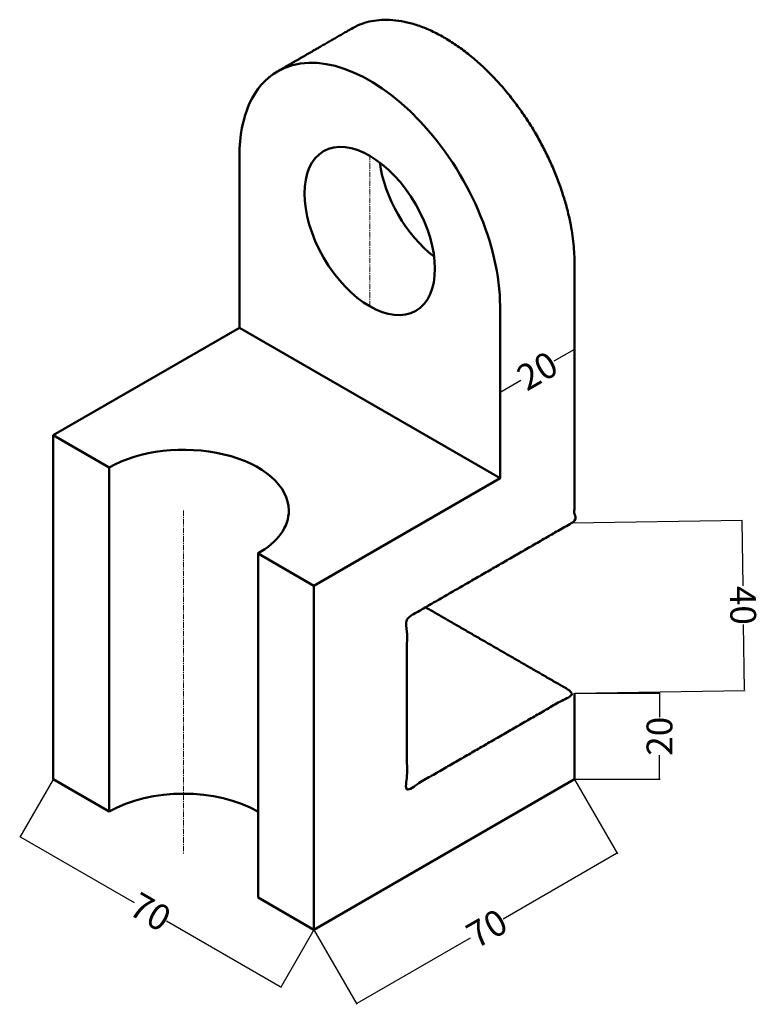
# Model space of a CAD drawing. Units: millimetres. Extents: x -6 to 166, y 11 to 240.
import ezdxf

# ---------------------------------------------------------------- set-up
doc = ezdxf.new("R2010")
doc.units = ezdxf.units.MM
doc.header["$MEASUREMENT"] = 0
doc.linetypes.add('CENTER', pattern=[2, 1.25, -0.25, 0.25, -0.25])
for name, color, linetype, lineweight in [('M-CNTR', 4, 'CENTER', 18), ('M-DIMS', 2, 'Continuous', 25), ('M-OUTL', 7, 'Continuous', 50)]:
    doc.layers.add(name, color=color, linetype=linetype, lineweight=lineweight)
doc.styles.get("Standard").update_dxf_attribs({"font": 'arial.ttf'})
doc.dimstyles.get("Standard").update_dxf_attribs({"dimtxt": 6, "dimasz": 0.18, "dimexe": 0.18, "dimexo": 0.0625, "dimgap": 0.09, "dimtad": 0, "dimtoh": 1, "dimdec": 0, "dimzin": 0, "dimdsep": 46, "dimtxsty": 'Standard', "dimcen": 0.09, "dimadec": 0, "dimazin": 0, "dimtfac": 1, "dimtdec": 0, "dimtofl": 0, "dimtmove": 0, "dimatfit": 3, "dimfxl": 1, "dimtolj": 1, "dimtzin": 0, "dimarcsym": 0})

# ---------------------------------------------------------------- blocks, each defined once
blk = doc.blocks.new('*D1')
at = {"layer": 'Defpoints', "color": 0, "transparency": 16777216}
for p in [(121.94, 122.99), (122.57, 83.35), (162.08, 83.99)]:
    blk.add_point(p, dxfattribs=at)
at = {"layer": 'M-DIMS', "color": 0, "lineweight": -2, "transparency": 16777216}
for p, q in [((122, 122.99), (161.63, 123.62)), ((161.45, 123.44), (161.69, 108.3)), ((162.08, 84.17), (161.84, 99.31)), ((122.64, 83.35), (162.26, 83.99))]:
    blk.add_line(p, q, dxfattribs=at)
at = {"layer": 'M-DIMS', "color": 0, "transparency": 16777216}
for points in [[(161.48, 123.44), (161.42, 123.44), (161.45, 123.62)], [(162.11, 84.17), (162.05, 84.17), (162.08, 83.99)]]:
    blk.add_solid(points, dxfattribs=at)
at = {"layer": 'M-DIMS', "color": 0, "transparency": 16777216, "insert": (161.76, 103.8), "char_height": 6, "attachment_point": 5, "rotation": 270.9187}
blk.add_mtext('\\A1;40', dxfattribs=at)
blk = doc.blocks.new('*D2')
at = {"layer": 'Defpoints', "color": 0, "transparency": 16777216}
for p in [(122.57, 83.35), (122.57, 63.35), (142.32, 63.35)]:
    blk.add_point(p, dxfattribs=at)
at = {"layer": 'M-DIMS', "color": 0, "lineweight": -2, "transparency": 16777216}
for p, q in [((122.64, 83.35), (142.5, 83.35)), ((142.32, 83.17), (142.32, 77.78)), ((142.32, 63.53), (142.32, 68.92)), ((122.64, 63.35), (142.5, 63.35))]:
    blk.add_line(p, q, dxfattribs=at)
at = {"layer": 'M-DIMS', "color": 0, "transparency": 16777216}
for points in [[(142.29, 83.17), (142.35, 83.17), (142.32, 83.35)], [(142.29, 63.53), (142.35, 63.53), (142.32, 63.35)]]:
    blk.add_solid(points, dxfattribs=at)
at = {"layer": 'M-DIMS', "color": 0, "transparency": 16777216, "insert": (142.32, 73.35), "char_height": 6, "attachment_point": 5, "rotation": 90}
blk.add_mtext('\\A1;20', dxfattribs=at)
blk = doc.blocks.new('*D3')
at = {"layer": 'Defpoints', "color": 0, "transparency": 16777216}
for p in [(122.57, 163.35), (122.57, 163.35), (105.25, 153.35)]:
    blk.add_point(p, dxfattribs=at)
at = {"layer": 'M-DIMS', "color": 0, "lineweight": -2, "transparency": 16777216}
for p, q in [((122.42, 163.26), (117.75, 160.57)), ((122.54, 163.41), (122.48, 163.51)), ((105.41, 153.44), (110.08, 156.14)), ((105.22, 153.41), (105.16, 153.51))]:
    blk.add_line(p, q, dxfattribs=at)
at = {"layer": 'M-DIMS', "color": 0, "transparency": 16777216}
for points in [[(122.4, 163.29), (122.43, 163.24), (122.57, 163.35)], [(105.39, 153.47), (105.42, 153.42), (105.25, 153.35)]]:
    blk.add_solid(points, dxfattribs=at)
at = {"layer": 'M-DIMS', "color": 0, "transparency": 16777216, "insert": (113.91, 158.35), "char_height": 6, "attachment_point": 5, "rotation": 30}
blk.add_mtext('\\A1;20', dxfattribs=at)
blk = doc.blocks.new('*D4')
at = {"layer": 'Defpoints', "color": 0, "transparency": 16777216}
for p in [(122.57, 63.35), (132.5, 46.17), (61.95, 28.35)]:
    blk.add_point(p, dxfattribs=at)
at = {"layer": 'M-DIMS', "color": 0, "lineweight": -2, "transparency": 16777216}
for p, q in [((122.6, 63.3), (132.59, 46.01)), ((132.34, 46.08), (105.95, 30.84)), ((61.98, 28.3), (71.96, 11.01)), ((72.03, 11.26), (98.41, 26.49))]:
    blk.add_line(p, q, dxfattribs=at)
at = {"layer": 'M-DIMS', "color": 0, "transparency": 16777216}
for points in [[(132.32, 46.1), (132.35, 46.05), (132.5, 46.17)], [(72.01, 11.28), (72.04, 11.23), (71.87, 11.17)]]:
    blk.add_solid(points, dxfattribs=at)
at = {"layer": 'M-DIMS', "color": 0, "transparency": 16777216, "insert": (102.18, 28.67), "char_height": 6, "attachment_point": 5, "rotation": 30}
blk.add_mtext('\\A1;70', dxfattribs=at)
blk = doc.blocks.new('*D5')
at = {"layer": 'Defpoints', "color": 0, "transparency": 16777216}
for p in [(1.33, 63.35), (61.95, 28.35), (54.25, 15.01)]:
    blk.add_point(p, dxfattribs=at)
at = {"layer": 'M-DIMS', "color": 0, "lineweight": -2, "transparency": 16777216}
for p, q in [((1.3, 63.3), (-6.46, 49.85)), ((-6.22, 49.92), (20.17, 34.69)), ((54.09, 15.1), (27.71, 30.33)), ((61.92, 28.3), (54.16, 14.85))]:
    blk.add_line(p, q, dxfattribs=at)
at = {"layer": 'M-DIMS', "color": 0, "transparency": 16777216}
for points in [[(-6.2, 49.95), (-6.23, 49.89), (-6.37, 50.01)], [(54.11, 15.13), (54.08, 15.07), (54.25, 15.01)]]:
    blk.add_solid(points, dxfattribs=at)
at = {"layer": 'M-DIMS', "color": 0, "transparency": 16777216, "insert": (23.94, 32.51), "char_height": 6, "attachment_point": 5, "rotation": 330}
blk.add_mtext('\\A1;70', dxfattribs=at)

msp = doc.modelspace()

# ---------------------------------------------------------------- linework, layer by layer
at = {"layer": 'M-CNTR'}
for p, q in [((74.94, 173.35), (74.94, 208.35)), ((31.64, 125.85), (31.64, 45.85))]:
    msp.add_line(p, q, dxfattribs=at)
at = {"layer": 'M-OUTL'}
for p, q in [((44.63, 168.35), (44.63, 208.35)), ((1.33, 143.35), (44.63, 168.35)), ((14.32, 135.85), (1.33, 143.35)), ((1.33, 63.35), (1.33, 143.35)), ((14.32, 55.85), (14.32, 135.85)), ((61.95, 108.35), (105.25, 133.35)), ((61.95, 108.35), (48.96, 115.85)), ((48.96, 35.85), (48.96, 115.85)), ((14.32, 55.85), (1.33, 63.35)), ((61.95, 28.35), (48.96, 35.85))]:
    msp.add_line(p, q, dxfattribs=at)
for points in [[(44.63, 168.35), (105.25, 133.35), (105.25, 173.35)], [(61.95, 108.35), (61.95, 28.35), (122.57, 63.35), (122.57, 83.35)]]:
    msp.add_lwpolyline(points, dxfattribs=at)
for centre, major_axis, start_param, end_param in [((74.94, 190.85), (21.43, -37.12), 0.785398, 3.141593), ((74.94, 190.85), (21.43, -37.12), 3.141593, 3.926991), ((92.26, 200.85), (10.72, -18.56), 4.082549, 5.342229), ((31.64, 125.85), (-24.49, 0), 3.141593, 5.497787), ((31.64, 125.85), (-24.49, 0), 2.356194, 3.141593), ((31.64, 45.85), (-24.49, 0), 3.926991, 5.497787)]:
    msp.add_ellipse(centre, major_axis=major_axis, ratio=0.57735, start_param=start_param, end_param=end_param, dxfattribs=at)
msp.add_ellipse((74.94, 190.85), major_axis=(10.72, -18.56), ratio=0.57735, dxfattribs=at)
msp.add_rational_spline([(87.93, 103.35), (105.25, 93.35), (122.57, 83.35), (103.09, 72.1), (83.6, 60.85), (83.6, 80.85), (83.6, 100.85), (103.09, 112.1), (122.57, 123.35), (122.57, 133.35), (122.57, 143.35), (122.57, 163.35), (122.57, 183.35), (122.57, 206.74), (103.86, 226.49), (85.15, 246.24), (70.83, 237.98), (62.17, 232.98), (53.51, 227.98)], [1, 1, 1, 1, 1, 1, 1, 1, 1, 1, 1, 1, 1, 0.831469612303, 1, 0.831469612303, 1, 1, 1], degree=2, knots=[0, 0, 0, 1, 1, 2, 2, 3, 3, 4, 4, 5, 5, 6, 6, 7.178097, 7.178097, 8.356194, 8.356194, 9.356194, 9.356194, 9.356194], dxfattribs=at)

# ---------------------------------------------------------------- dimensions: what is measured, and where the dimension line sits
at = {"layer": 'M-DIMS'}
for p1, p2, distance, picture, middle in [((105.25, 153.35), (122.57, 163.35), 0, '*D3', (113.91, 158.35)), ((121.94, 122.99), (122.57, 83.35), 39.51, '*D1', (161.76, 103.8)), ((122.57, 83.35), (122.57, 63.35), 19.74, '*D2', (142.32, 73.35)), ((1.33, 63.35), (61.95, 28.35), -15.41, '*D5', (23.94, 32.51)), ((61.95, 28.35), (122.57, 63.35), -19.84, '*D4', (102.18, 28.67))]:
    dim = msp.add_aligned_dim(p1=p1, p2=p2, distance=distance, dimstyle='Standard', override={"dimclrd": 0, "dimclre": 0, "dimclrt": 0}, dxfattribs=at)
    dim.commit()
    dim.dimension.update_dxf_attribs({"geometry": picture, "text_midpoint": middle})

doc.saveas('drawing.dxf')
